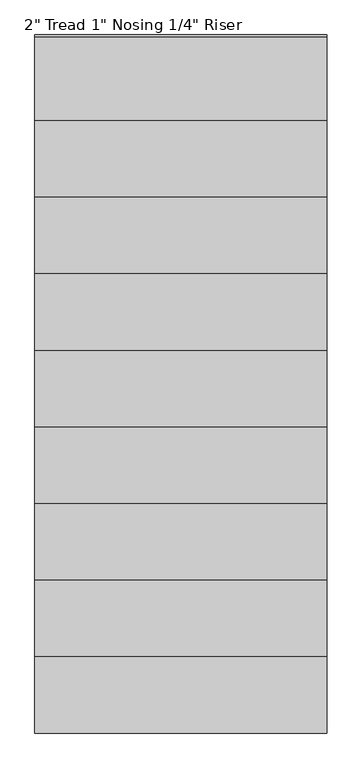
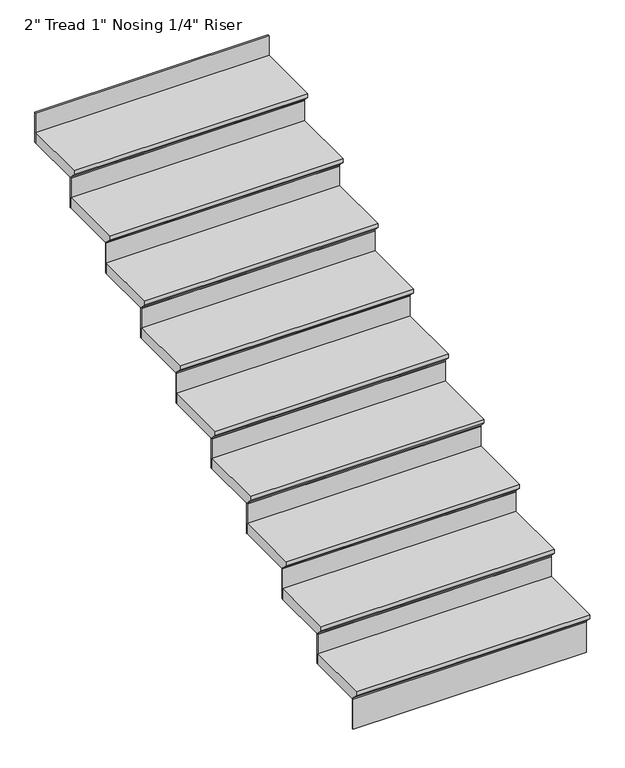
"""IFC4 building model written with IfcOpenShell, lengths in millimetres: stair flight geometry."""

from ifc_helpers import new_model, si_unit, frame, origin, place, context, project, spatial, polyline, outline, extrude, source, transform, mapped, element, save


def stair_flight_df8bf18d(model_context):
    return source(origin(), model_context, "Body", "SweptSolid", [
        extrude(outline(polyline([(9995.9922903, 1600.2), (10300.7922903, 1600.2), (10300.7922903, 1549.4), (10021.3922903, 1549.4), (10021.3922903, 1555.75), (9995.9922903, 1581.15), (9995.9922903, 1600.2)])), frame((-17359.2847893, 0.0, 0.0), z_axis=(1.0, 0.0, 0.0), x_axis=(0.0, 1.0, 0.0)), (0.0, 0.0, 1.0), 1066.8),
        extrude(outline(polyline([(-16292.4847893, 10027.7422903), (-16292.4847893, 10021.3922903), (-17359.2847893, 10021.3922903), (-17359.2847893, 10027.7422903), (-16292.4847893, 10027.7422903)])), frame((0.0, 0.0, 1403.9272727), z_axis=(0.0, 0.0, 1.0), x_axis=(1.0, 0.0, 0.0)), (0.0, 0.0, 1.0), 145.4727273),
        extrude(outline(polyline([(-16292.4847893, 10307.1422903), (-16292.4847893, 10300.7922903), (-17359.2847893, 10300.7922903), (-17359.2847893, 10307.1422903), (-16292.4847893, 10307.1422903)])), frame((0.0, 0.0, 1549.4), z_axis=(0.0, 0.0, 1.0), x_axis=(1.0, 0.0, 0.0)), (0.0, 0.0, 1.0), 145.4727273),
        extrude(outline(polyline([(10275.3922903, 1745.6727273), (10580.1922903, 1745.6727273), (10580.1922903, 1694.8727273), (10300.7922903, 1694.8727273), (10300.7922903, 1701.2227273), (10275.3922903, 1726.6227273), (10275.3922903, 1745.6727273)])), frame((-17359.2847893, 0.0, 0.0), z_axis=(1.0, 0.0, 0.0), x_axis=(0.0, 1.0, 0.0)), (0.0, 0.0, 1.0), 1066.8),
        extrude(outline(polyline([(-16292.4847893, 10586.5422903), (-16292.4847893, 10580.1922903), (-17359.2847893, 10580.1922903), (-17359.2847893, 10586.5422903), (-16292.4847893, 10586.5422903)])), frame((0.0, 0.0, 1694.8727273), z_axis=(0.0, 0.0, 1.0), x_axis=(1.0, 0.0, 0.0)), (0.0, 0.0, 1.0), 145.4727273),
        extrude(outline(polyline([(10554.7922903, 1891.1454545), (10859.5922903, 1891.1454545), (10859.5922903, 1840.3454545), (10580.1922903, 1840.3454545), (10580.1922903, 1846.6954545), (10554.7922903, 1872.0954545), (10554.7922903, 1891.1454545)])), frame((-17359.2847893, 0.0, 0.0), z_axis=(1.0, 0.0, 0.0), x_axis=(0.0, 1.0, 0.0)), (0.0, 0.0, 1.0), 1066.8),
        extrude(outline(polyline([(-16292.4847893, 10865.9422903), (-16292.4847893, 10859.5922903), (-17359.2847893, 10859.5922903), (-17359.2847893, 10865.9422903), (-16292.4847893, 10865.9422903)])), frame((0.0, 0.0, 1840.3454545), z_axis=(0.0, 0.0, 1.0), x_axis=(1.0, 0.0, 0.0)), (0.0, 0.0, 1.0), 145.4727273),
        extrude(outline(polyline([(10834.1922903, 2036.6181818), (11138.9922903, 2036.6181818), (11138.9922903, 1985.8181818), (10859.5922903, 1985.8181818), (10859.5922903, 1992.1681818), (10834.1922903, 2017.5681818), (10834.1922903, 2036.6181818)])), frame((-17359.2847893, 0.0, 0.0), z_axis=(1.0, 0.0, 0.0), x_axis=(0.0, 1.0, 0.0)), (0.0, 0.0, 1.0), 1066.8),
        extrude(outline(polyline([(-16292.4847893, 11145.3422903), (-16292.4847893, 11138.9922903), (-17359.2847893, 11138.9922903), (-17359.2847893, 11145.3422903), (-16292.4847893, 11145.3422903)])), frame((0.0, 0.0, 1985.8181818), z_axis=(0.0, 0.0, 1.0), x_axis=(1.0, 0.0, 0.0)), (0.0, 0.0, 1.0), 145.4727273),
        extrude(outline(polyline([(11113.5922903, 2182.0909091), (11418.3922903, 2182.0909091), (11418.3922903, 2131.2909091), (11138.9922903, 2131.2909091), (11138.9922903, 2137.6409091), (11113.5922903, 2163.0409091), (11113.5922903, 2182.0909091)])), frame((-17359.2847893, 0.0, 0.0), z_axis=(1.0, 0.0, 0.0), x_axis=(0.0, 1.0, 0.0)), (0.0, 0.0, 1.0), 1066.8),
        extrude(outline(polyline([(-16292.4847893, 11424.7422903), (-16292.4847893, 11418.3922903), (-17359.2847893, 11418.3922903), (-17359.2847893, 11424.7422903), (-16292.4847893, 11424.7422903)])), frame((0.0, 0.0, 2131.2909091), z_axis=(0.0, 0.0, 1.0), x_axis=(1.0, 0.0, 0.0)), (0.0, 0.0, 1.0), 145.4727273),
        extrude(outline(polyline([(11392.9922903, 2327.5636364), (11697.7922903, 2327.5636364), (11697.7922903, 2276.7636364), (11418.3922903, 2276.7636364), (11418.3922903, 2283.1136364), (11392.9922903, 2308.5136364), (11392.9922903, 2327.5636364)])), frame((-17359.2847893, 0.0, 0.0), z_axis=(1.0, 0.0, 0.0), x_axis=(0.0, 1.0, 0.0)), (0.0, 0.0, 1.0), 1066.8),
        extrude(outline(polyline([(-16292.4847893, 11704.1422903), (-16292.4847893, 11697.7922903), (-17359.2847893, 11697.7922903), (-17359.2847893, 11704.1422903), (-16292.4847893, 11704.1422903)])), frame((0.0, 0.0, 2276.7636364), z_axis=(0.0, 0.0, 1.0), x_axis=(1.0, 0.0, 0.0)), (0.0, 0.0, 1.0), 145.4727273),
        extrude(outline(polyline([(11672.3922903, 2473.0363636), (11977.1922903, 2473.0363636), (11977.1922903, 2422.2363636), (11697.7922903, 2422.2363636), (11697.7922903, 2428.5863636), (11672.3922903, 2453.9863636), (11672.3922903, 2473.0363636)])), frame((-17359.2847893, 0.0, 0.0), z_axis=(1.0, 0.0, 0.0), x_axis=(0.0, 1.0, 0.0)), (0.0, 0.0, 1.0), 1066.8),
        extrude(outline(polyline([(-16292.4847893, 11983.5422903), (-16292.4847893, 11977.1922903), (-17359.2847893, 11977.1922903), (-17359.2847893, 11983.5422903), (-16292.4847893, 11983.5422903)])), frame((0.0, 0.0, 2422.2363636), z_axis=(0.0, 0.0, 1.0), x_axis=(1.0, 0.0, 0.0)), (0.0, 0.0, 1.0), 145.4727273),
        extrude(outline(polyline([(11951.7922903, 2618.5090909), (12256.5922903, 2618.5090909), (12256.5922903, 2567.7090909), (11977.1922903, 2567.7090909), (11977.1922903, 2574.0590909), (11951.7922903, 2599.4590909), (11951.7922903, 2618.5090909)])), frame((-17359.2847893, 0.0, 0.0), z_axis=(1.0, 0.0, 0.0), x_axis=(0.0, 1.0, 0.0)), (0.0, 0.0, 1.0), 1066.8),
        extrude(outline(polyline([(-16292.4847893, 12262.9422903), (-16292.4847893, 12256.5922903), (-17359.2847893, 12256.5922903), (-17359.2847893, 12262.9422903), (-16292.4847893, 12262.9422903)])), frame((0.0, 0.0, 2567.7090909), z_axis=(0.0, 0.0, 1.0), x_axis=(1.0, 0.0, 0.0)), (0.0, 0.0, 1.0), 145.4727273),
        extrude(outline(polyline([(-16292.4847893, 12542.3422903), (-16292.4847893, 12535.9922903), (-17359.2847893, 12535.9922903), (-17359.2847893, 12542.3422903), (-16292.4847893, 12542.3422903)])), frame((0.0, 0.0, 2713.1818182), z_axis=(0.0, 0.0, 1.0), x_axis=(1.0, 0.0, 0.0)), (0.0, 0.0, 1.0), 145.4727273),
        extrude(outline(polyline([(12231.1922903, 2763.9818182), (12535.9922903, 2763.9818182), (12535.9922903, 2713.1818182), (12256.5922903, 2713.1818182), (12256.5922903, 2719.5318182), (12231.1922903, 2744.9318182), (12231.1922903, 2763.9818182)])), frame((-17359.2847893, 0.0, 0.0), z_axis=(1.0, 0.0, 0.0), x_axis=(0.0, 1.0, 0.0)), (0.0, 0.0, 1.0), 1066.8),
    ])


if __name__ == "__main__":
    model = new_model("IFC4")
    model_context = context("Model", 3, world=origin())
    ifc_project = project(units=[si_unit("LENGTHUNIT", "METRE", prefix="MILLI")], contexts=[model_context])
    site = spatial("IfcSite", under=ifc_project)
    building = spatial("IfcBuilding", under=site)
    placement = place(None, origin())
    stair_flight_shape = stair_flight_df8bf18d(model_context)
    element("IfcStairFlight", 1, ObjectType="2\" Tread 1\" Nosing 1/4\" Riser", at=placement, inside=building, context=model_context, shape_type="MappedRepresentation", body=[
        mapped(stair_flight_shape, transform((0.0, 0.0, 0.0), x_axis=(1.0, 0.0, 0.0), y_axis=(0.0, 1.0, 0.0), z_axis=(0.0, 0.0, 1.0))),
    ])
    save(model, "model.ifc")
